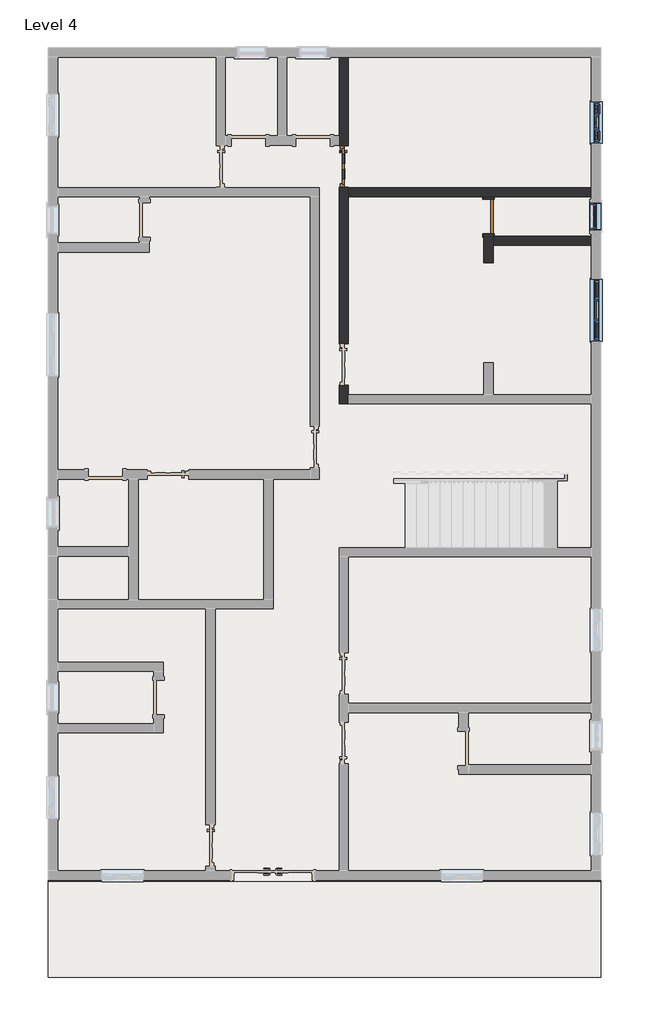
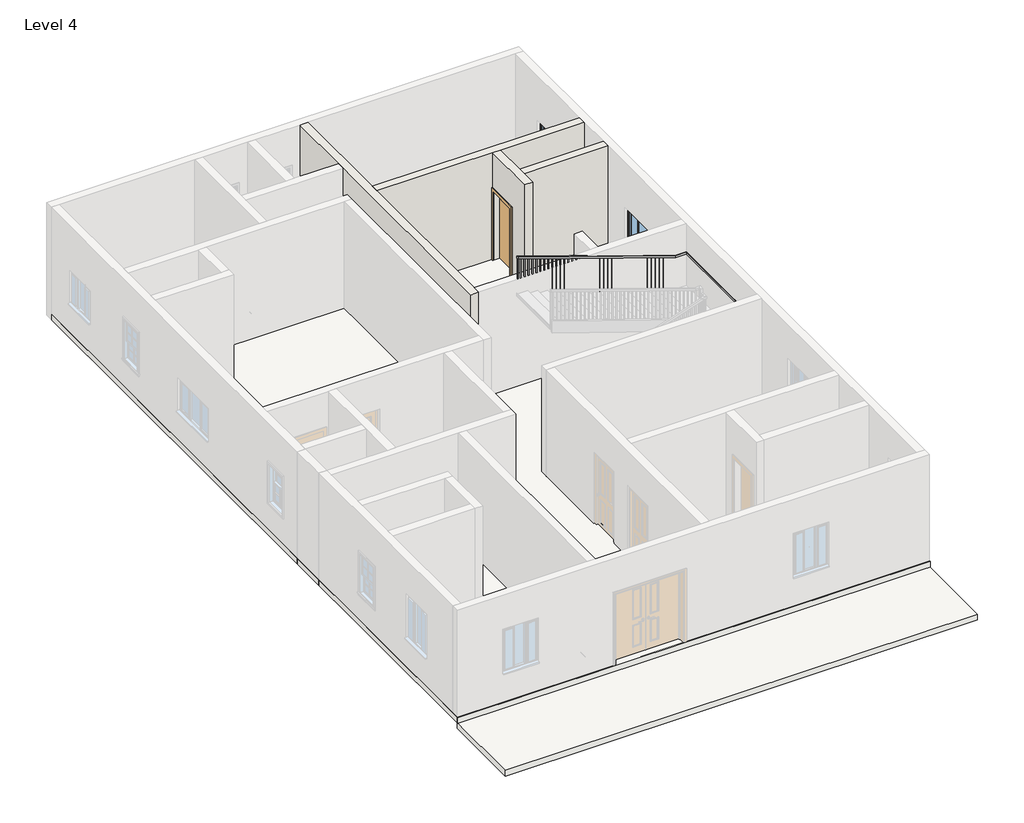
# One storey, part 2 of 3: 4 roofs, 4 walls, 3 windows, 2 doors, 1 railing, 1 slab.
# Revit data of these elements (continued)
# Type "Windows_Tpl_Plain : 1360x910mm" (continued)
#   Material Trim = Window Frame
#   Material Glass = Glass
#   Material Frame = Window Frame
#   Wall Closure = (empty or 0)
# Type "Windows_Tpl_w-Glazing_Cross-Bars : 910x910mm"
#   Type Mark = "24"
#   Operation = "TriplePanelVertical"
#   Construction Type Id = "GSP4R"
#   Manufacturer = "Revit"
#   Keynote = "L10"
#   Analytic Construction = "1/8 in Pilkington single glazing"
#   Wrap Layers (Ext) from Ext = 0' - 4.03543"
#   Wrap Layers (Int) from Ext = 0' - 6.98819"
#   Window Board Projection = 0' - 0.98425"
#   Window Board Extension = 0' - 0.98425"
#   Visual Light Transmittance = 0.9
#   Solar Heat Gain Coefficient = 0.78
#   Rough Width = 2' - 11.82677"
#   Rough Height = 2' - 11.82677"
#   Height = 2' - 11.82677"
#   Width = 2' - 11.82677"
#   Heat Transfer Coefficient (U) = 0.6496 BTU/(h·ft²·°F)
#   Glazing Thickness = 0' - 0.94488"
#   Glazing Bar Thickness = 0' - 0.7874"
#   FrameOffset - External = 0' - 1.9685"
#   Frame Depth = 0' - 2.55906"
#   Default Head Height = 6' - 11.07087"
#   Cill Depth = 0' - 3.44488"
#   Cavity Closer Width = 0' - 1.9685"
#   Cavity Closer Offset from Ext = 0' - 4.03543"
#   Cavity Closer Depth = 0' - 3.34646"
#   Vis - Glazing Bars = yes
#   Vis - Cavity Closers = yes
#   Define Thermal Properties by = 1
#   Material Trim = Window Frame
#   Material Glazing Bars = Window Frame
#   Material Glass = Glass
#   Material Frame = Window Frame
#   Wall Closure = (empty or 0)
# Element 1 (IfcDoor, "Doors_ExtSgl_2 : 2'x7\"")
#   Phase Created = New Construction
#   Materials on its faces: "Door - Panel", "Door - Handle", "Door - Frame/Mullion", "Door - Glazing"
# Element 2 (IfcDoor, "Single-Flush : 30\" x 80\"")
#   Phase Created = New Construction
#   Materials on its faces: "Door - Frame", "Door - Panel"
# Element 3 (IfcRailing, "Handrail - Rectangular")
#   Phase Created = New Construction
# Elements 4, 5, 6, 7 (IfcRoof, "Generic - 12\"")
#   built-in parameter 1001705 = 30.5 (stored number, unit not read)
#   built-in parameter 1001710 = 33615
#   Phase Created = New Construction
#   Materials on its faces: "Default Roof"
# Element 8 (IfcSlab, "Generic - 12\"")
#   Height Offset From Level = 0' - 0"
#   Phase Created = New Construction
#   Materials on its faces: "Default Floor"
# Elements 9, 10, 11, 12 (IfcWall, "Generic - 4.5\" p")
#   Top Offset = 0' - 0"
#   Base Offset = 0' - 0"
#   Unconnected Height = 10' - 0"
#   wall height = 10' - 0"
#   Phase Created = New Construction
#   Base Constraint = Level 4
#   Materials on its faces: "Default Wall"
# Element 13 (IfcWindow, "Window-Double-Hung : 24\" x 42\"")
#   Mark = "45"
#   Window Inset = 0' - 0"
#   Interior Wall Closure = 0' - 1 1/2"
#   Frame Extension = 0' - 1 1/4"
#   Exterior Wall Closure = 0' - 0 1/2"
#   Interior Trim Visibility = yes
#   Indicator Visibility = yes
#   Exterior Trim Visibility = yes
#   Phase Created = New Construction
#   Materials on its faces: "Wood - Stained", "Glass", "Clad - White"
# Element 14 (IfcWindow, "Windows_Tpl_Plain : 1360x910mm")
#   Mark = "38"
#   Phase Created = New Construction
#   Materials on its faces: "Window Frame", "Glass"
# Element 15 (IfcWindow, "Windows_Tpl_w-Glazing_Cross-Bars : 910x910mm")
#   Mark = "41"
#   Phase Created = New Construction
#   Materials on its faces: "Window Frame", "Glass"
# Materials
#   "Door - Glazing": colour RGB 0 0 255, transparency 0.75
#   "Door - Panel": class "Wood", colour RGB 210 159 95, transparency 0, Cost = 0
#   "Door - Frame/Mullion": class "Wood", colour RGB 212 179 113, transparency 0
#   "Door - Handle": colour RGB 246 240 166, transparency 0
#   "Door - Frame": colour RGB 118 70 51, transparency 0, Cost = 0
#   "Wood - Stained": class "Wood", colour RGB 224 178 126, transparency 0, Cost = 0
#   "Clad - White": class "Wood", colour RGB 242 242 238, transparency 0, Cost = 0
#   "Glass": class "Glass", colour RGB 0 128 192, transparency 0.75, Description = "Soda Lime Glass", Cost = 0
#   "Window Frame": colour RGB 249 249 249, transparency 0
#   "Default Roof": colour RGB 88 101 114, transparency 0, Cost = 0
#   "Default Floor": colour RGB 128 128 128, transparency 0, Cost = 0
#   "Default Wall": colour RGB 128 128 128, transparency 0, Cost = 0
